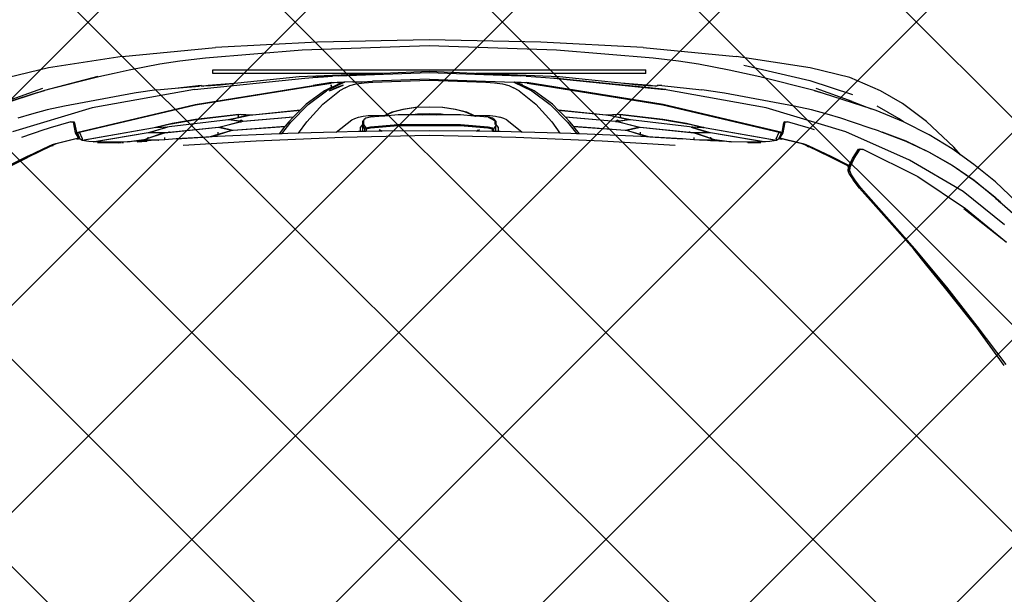
# Model space of a CAD drawing. Units: inches. Extents: x 2167 to 2589, y 1680 to 2489.
# Tile 27 of 38: x 2356 to 2389, y 1815 to 1835. Entities that reach past the tile are written whole.
import ezdxf

# ---------------------------------------------------------------- set-up
doc = ezdxf.new("R2010")
doc.units = ezdxf.units.IN
doc.header["$MEASUREMENT"] = 0
doc.layers.get('0').update_dxf_attribs({"color": 250})
doc.layers.add('C-PRKG-VEHS', color=8, linetype='Continuous', lineweight=13)
doc.layers.add('L-PVMT-PATT', color=252, linetype='Continuous', lineweight=13)
doc.layers.add('Edges', color=250, linetype='Continuous')

# ---------------------------------------------------------------- blocks, each defined once
blk = doc.blocks.new('Nissan Qashqai pl')
at = {"layer": 'Edges'}
for p, q in [((7.4801, 12.6274), (7.4565, 12.6023)), ((7.4827, 12.6103), (7.5001, 12.6302)), ((7.5081, 12.6131), (7.4679, 12.5634)), ((7.4884, 12.5664), (7.5289, 12.6158)), ((7.5243, 12.6101), (7.5286, 12.6146)), ((7.676, 12.6152), (7.6296, 12.5803)), ((7.6769, 12.6129), (7.6306, 12.5791)), ((7.4565, 12.6023), (7.4354, 12.5766)), ((7.4542, 12.5765), (7.4744, 12.6015)), ((7.475, 12.6016), (7.4549, 12.5767)), ((7.4744, 12.6015), (7.4804, 12.6079)), ((7.4762, 12.6028), (7.475, 12.6016)), ((7.4752, 12.6016), (7.4762, 12.6028)), ((7.4762, 12.6028), (7.478, 12.6049)), ((7.4804, 12.6079), (7.478, 12.6049)), ((7.478, 12.6049), (7.479, 12.6061)), ((7.479, 12.6061), (7.4815, 12.6089)), ((7.479, 12.6061), (7.4801, 12.6074)), ((7.4801, 12.6074), (7.4804, 12.6079)), ((7.4804, 12.6079), (7.4807, 12.6082)), ((7.4804, 12.6079), (7.4804, 12.6079)), ((7.4807, 12.6082), (7.4821, 12.6097)), ((7.4815, 12.6089), (7.4821, 12.6097)), ((7.4821, 12.6097), (7.4827, 12.6103)), ((7.4882, 12.5645), (7.5243, 12.6101)), ((7.4354, 12.5766), (7.4239, 12.5604)), ((7.4363, 12.5502), (7.4542, 12.5765)), ((7.4549, 12.5767), (7.4369, 12.5504)), ((7.6296, 12.5803), (7.5827, 12.5441)), ((7.6301, 12.5787), (7.618, 12.5691)), ((7.6306, 12.5791), (7.6301, 12.5787)), ((7.4498, 12.5093), (7.4884, 12.5664)), ((7.618, 12.5691), (7.5829, 12.5411)), ((7.618, 12.5691), (7.584, 12.5429)), ((7.4147, 12.5524), (7.3837, 12.5197)), ((7.4239, 12.5604), (7.4147, 12.5524)), ((7.4239, 12.5604), (7.4166, 12.5503)), ((7.4679, 12.5634), (7.4302, 12.4993)), ((7.4166, 12.5503), (7.3997, 12.5227)), ((7.4205, 12.5229), (7.4363, 12.5502)), ((7.4369, 12.5504), (7.4211, 12.5232)), ((7.5827, 12.5441), (7.5369, 12.5057)), ((7.584, 12.5429), (7.5568, 12.5201)), ((7.5829, 12.5411), (7.5568, 12.5201)), ((7.3837, 12.5197), (7.3624, 12.4907)), ((7.3997, 12.5227), (7.3845, 12.4925)), ((7.4071, 12.4948), (7.4205, 12.5229)), ((7.4211, 12.5232), (7.4078, 12.4951)), ((7.5568, 12.5201), (7.5371, 12.5042)), ((7.4172, 12.4431), (7.4498, 12.5093)), ((7.5369, 12.5057), (7.4635, 12.4408)), ((7.3962, 12.466), (7.4071, 12.4948)), ((7.4302, 12.4993), (7.3963, 12.4227)), ((7.4078, 12.4951), (7.3969, 12.4665)), ((7.4638, 12.439), (7.5371, 12.5042)), ((7.3624, 12.4907), (7.347, 12.4644)), ((7.3805, 12.4866), (7.3655, 12.4604)), ((7.3843, 12.492), (7.3707, 12.4592)), ((7.3843, 12.492), (7.3805, 12.4866)), ((7.3845, 12.4925), (7.3843, 12.492)), ((7.347, 12.4644), (7.3309, 12.4276)), ((7.3707, 12.4592), (7.3688, 12.4532)), ((7.3938, 12.4583), (7.3925, 12.4542)), ((7.3951, 12.462), (7.3938, 12.4583)), ((7.3965, 12.4655), (7.3951, 12.462)), ((7.3965, 12.4655), (7.3962, 12.466)), ((7.3969, 12.4665), (7.3965, 12.4655)), ((7.3968, 12.4649), (7.3967, 12.4651)), ((7.3688, 12.4532), (7.3467, 12.3846)), ((7.3596, 12.4302), (7.3688, 12.4532)), ((7.3925, 12.4542), (7.3845, 12.4306)), ((7.4167, 12.4393), (7.4169, 12.4406)), ((7.4167, 12.4393), (7.4172, 12.4395)), ((7.417, 12.4377), (7.4167, 12.4393)), ((7.4169, 12.4412), (7.4172, 12.4431)), ((7.4169, 12.4406), (7.4172, 12.4423)), ((7.4169, 12.4406), (7.4169, 12.4412)), ((7.4169, 12.4398), (7.4169, 12.4406)), ((7.4282, 12.4328), (7.4169, 12.4398)), ((7.4172, 12.4395), (7.4169, 12.4398)), ((7.4283, 12.4307), (7.417, 12.4377)), ((7.4172, 12.4423), (7.4174, 12.4429)), ((7.4183, 12.4382), (7.4172, 12.4395)), ((7.4175, 12.4429), (7.4174, 12.4429)), ((7.4183, 12.4382), (7.4296, 12.4312)), ((7.4635, 12.4408), (7.4541, 12.4333)), ((7.4638, 12.439), (7.4541, 12.4313)), ((7.3309, 12.4276), (7.3193, 12.3797)), ((7.3345, 12.3793), (7.3514, 12.4308)), ((7.3596, 12.4302), (7.344, 12.3869)), ((7.3963, 12.4227), (7.3676, 12.3269)), ((7.3845, 12.4306), (7.3799, 12.4164)), ((7.4255, 12.4044), (7.4367, 12.4268)), ((7.4365, 12.4235), (7.4267, 12.4041)), ((7.4387, 12.428), (7.4282, 12.4328)), ((7.4359, 12.4272), (7.4283, 12.4307)), ((7.4383, 12.4272), (7.4296, 12.4312)), ((7.4367, 12.4268), (7.4359, 12.4272)), ((7.4378, 12.4261), (7.4365, 12.4235)), ((7.4365, 12.4235), (7.4365, 12.4235)), ((7.4367, 12.4268), (7.4383, 12.4272)), ((7.4379, 12.4263), (7.4378, 12.4261)), ((7.4379, 12.4263), (7.4383, 12.4272)), ((7.4379, 12.4263), (7.4389, 12.4269)), ((7.4384, 12.426), (7.4379, 12.4263)), ((7.4384, 12.426), (7.438, 12.4251)), ((7.4383, 12.4272), (7.4389, 12.4269)), ((7.4389, 12.4269), (7.4384, 12.426)), ((7.4387, 12.4259), (7.4384, 12.426)), ((7.4431, 12.4276), (7.4387, 12.428)), ((7.443, 12.4254), (7.4387, 12.4259)), ((7.44, 12.4264), (7.4389, 12.4269)), ((7.44, 12.4264), (7.4442, 12.4258)), ((7.4477, 12.427), (7.443, 12.4254)), ((7.4479, 12.4293), (7.4431, 12.4276)), ((7.4442, 12.4258), (7.4477, 12.427)), ((7.4477, 12.427), (7.4541, 12.4313)), ((7.4541, 12.4333), (7.4479, 12.4293)), ((7.3799, 12.4164), (7.375, 12.4)), ((7.375, 12.4), (7.3699, 12.3813)), ((7.4131, 12.3783), (7.4255, 12.4044)), ((7.4267, 12.4041), (7.4139, 12.3778)), ((7.3467, 12.3846), (7.3489, 12.3925)), ((7.3193, 12.3797), (7.3059, 12.291)), ((7.3161, 12.3001), (7.3345, 12.3793)), ((7.3467, 12.3846), (7.33, 12.3192)), ((7.3699, 12.3813), (7.3653, 12.3604)), ((7.3913, 12.3774), (7.3844, 12.3526)), ((7.3913, 12.3774), (7.3914, 12.3775)), ((7.3925, 12.3813), (7.3914, 12.3775)), ((7.3937, 12.3851), (7.3925, 12.3813)), ((7.4115, 12.3746), (7.4131, 12.3783)), ((7.4139, 12.3778), (7.4122, 12.3742)), ((7.4133, 12.3759), (7.4142, 12.3776)), ((7.4033, 12.3435), (7.4101, 12.3708)), ((7.4108, 12.3703), (7.4042, 12.3435)), ((7.4101, 12.3708), (7.4115, 12.3746)), ((7.4122, 12.3742), (7.4108, 12.3703)), ((7.3653, 12.3604), (7.3497, 12.2767)), ((7.3841, 12.3485), (7.3844, 12.3526)), ((7.3971, 12.3461), (7.3635, 12.2033)), ((7.364, 12.2029), (7.3968, 12.3424)), ((7.3846, 12.3495), (7.3841, 12.3485)), ((7.3841, 12.3485), (7.3853, 12.3483)), ((7.3846, 12.3495), (7.3976, 12.347)), ((7.3971, 12.3461), (7.3853, 12.3483)), ((7.3968, 12.3424), (7.398, 12.3449)), ((7.4046, 12.3389), (7.3968, 12.3424)), ((7.3983, 12.3458), (7.3971, 12.3461)), ((7.3976, 12.347), (7.4026, 12.3439)), ((7.398, 12.3449), (7.3999, 12.344)), ((7.398, 12.3449), (7.4012, 12.3441)), ((7.4012, 12.3441), (7.3983, 12.3458)), ((7.3999, 12.344), (7.4051, 12.3415)), ((7.3999, 12.344), (7.4048, 12.3417)), ((7.4033, 12.3427), (7.4012, 12.3441)), ((7.4012, 12.3441), (7.4015, 12.344)), ((7.4015, 12.344), (7.4028, 12.3437)), ((7.4026, 12.3439), (7.4033, 12.3435)), ((7.4033, 12.3435), (7.4042, 12.3422)), ((7.4042, 12.3422), (7.4033, 12.3427)), ((7.4042, 12.3435), (7.404, 12.3429)), ((7.404, 12.3429), (7.4043, 12.3428)), ((7.404, 12.3429), (7.4043, 12.3425)), ((7.4041, 12.3435), (7.4042, 12.3435)), ((7.4042, 12.3435), (7.4045, 12.3434)), ((7.4042, 12.3422), (7.4043, 12.3425)), ((7.4044, 12.3422), (7.4042, 12.3422)), ((7.4043, 12.3428), (7.4045, 12.3434)), ((7.4043, 12.3428), (7.4046, 12.3425)), ((7.4043, 12.3425), (7.4043, 12.3428)), ((7.4043, 12.3425), (7.4044, 12.3422)), ((7.4044, 12.3422), (7.4046, 12.3419)), ((7.4046, 12.3422), (7.4044, 12.3422)), ((7.4045, 12.3434), (7.405, 12.3456)), ((7.4045, 12.3434), (7.4048, 12.3433)), ((7.4046, 12.3425), (7.4047, 12.3424)), ((7.4047, 12.3424), (7.4046, 12.3422)), ((7.4046, 12.3422), (7.4046, 12.3419)), ((7.4048, 12.3422), (7.4046, 12.3422)), ((7.4046, 12.3419), (7.405, 12.3419)), ((7.4048, 12.3417), (7.4046, 12.3419)), ((7.4047, 12.3424), (7.4048, 12.3422)), ((7.4048, 12.3422), (7.405, 12.3419)), ((7.4048, 12.3417), (7.4052, 12.3416)), ((7.4051, 12.3415), (7.4048, 12.3417)), ((7.405, 12.3419), (7.4052, 12.3416)), ((7.4051, 12.3415), (7.4052, 12.3415)), ((7.4052, 12.3416), (7.4052, 12.3415)), ((7.4052, 12.3415), (7.4063, 12.3395)), ((7.4062, 12.3389), (7.4063, 12.3395)), ((7.4063, 12.3395), (7.4065, 12.3392)), ((7.3916, 12.2547), (7.4062, 12.3389)), ((7.4065, 12.3392), (7.3917, 12.2547)), ((7.4046, 12.3389), (7.4062, 12.3389)), ((7.4065, 12.3392), (7.4066, 12.3389)), ((7.4066, 12.3389), (7.408, 12.3313)), ((7.408, 12.3313), (7.4083, 12.3258)), ((7.33, 12.3192), (7.3261, 12.3009)), ((7.3676, 12.3269), (7.3455, 12.2042)), ((7.3971, 12.2599), (7.4083, 12.3258)), ((7.4084, 12.3244), (7.3975, 12.2599)), ((7.4083, 12.3258), (7.4084, 12.3244)), ((7.4084, 12.3244), (7.4087, 12.3195)), ((7.4087, 12.3195), (7.4087, 12.3037)), ((7.4092, 12.3184), (7.4091, 12.3206)), ((7.4092, 12.305), (7.4092, 12.3184)), ((7.3261, 12.3009), (7.3223, 12.2825)), ((7.4087, 12.3037), (7.4081, 12.2848)), ((7.2951, 12.1791), (7.3059, 12.291)), ((7.3223, 12.2825), (7.3186, 12.2641)), ((7.4054, 12.2651), (7.4081, 12.2848)), ((7.4081, 12.2838), (7.4079, 12.2798)), ((7.4081, 12.2848), (7.4081, 12.2838)), ((7.3494, 12.2741), (7.3457, 12.2495)), ((7.3498, 12.2768), (7.3494, 12.2741)), ((7.3497, 12.2767), (7.3494, 12.2741)), ((7.4079, 12.2798), (7.4059, 12.2651)), ((7.4079, 12.2798), (7.4069, 12.2598)), ((7.3186, 12.2641), (7.3149, 12.2457)), ((7.391, 12.2387), (7.3967, 12.2579)), ((7.3969, 12.257), (7.3965, 12.256)), ((7.3967, 12.2579), (7.3971, 12.2599)), ((7.3968, 12.2559), (7.3969, 12.257)), ((7.3975, 12.2599), (7.3973, 12.258)), ((7.3973, 12.258), (7.3977, 12.2439)), ((7.4048, 12.2612), (7.3982, 12.2419)), ((7.3983, 12.244), (7.4038, 12.2599)), ((7.4028, 12.2599), (7.4038, 12.2599)), ((7.4038, 12.2599), (7.4049, 12.2631)), ((7.4053, 12.2622), (7.4048, 12.2612)), ((7.4049, 12.2631), (7.4054, 12.2651)), ((7.4053, 12.2612), (7.4053, 12.2622)), ((7.4061, 12.2473), (7.4053, 12.2612)), ((7.4059, 12.2618), (7.4056, 12.2621)), ((7.4059, 12.2651), (7.4058, 12.2632)), ((7.4058, 12.2632), (7.4059, 12.2618)), ((7.4059, 12.2618), (7.4064, 12.2523)), ((7.4069, 12.2598), (7.4064, 12.2523)), ((7.3149, 12.2457), (7.3113, 12.2217)), ((7.3407, 12.2016), (7.3457, 12.2495)), ((7.3909, 12.2508), (7.3864, 12.231)), ((7.3869, 12.2347), (7.3912, 12.2527)), ((7.3901, 12.2368), (7.391, 12.2507)), ((7.3914, 12.2527), (7.3906, 12.2386)), ((7.3908, 12.2366), (7.3965, 12.256)), ((7.3911, 12.2518), (7.3909, 12.2508)), ((7.391, 12.2507), (7.3911, 12.2518)), ((7.3912, 12.2517), (7.3911, 12.2518)), ((7.3912, 12.2527), (7.3916, 12.2547)), ((7.3917, 12.2547), (7.3914, 12.2527)), ((7.3972, 12.2421), (7.3968, 12.2559)), ((7.4061, 12.2472), (7.4057, 12.24)), ((7.4064, 12.2523), (7.4061, 12.2473)), ((7.4061, 12.2472), (7.4061, 12.2473)), ((7.3813, 12.2021), (7.3869, 12.2347)), ((7.3815, 12.1638), (7.3899, 12.2348)), ((7.3903, 12.2347), (7.382, 12.1639)), ((7.3899, 12.2348), (7.3901, 12.2368)), ((7.3908, 12.2366), (7.3903, 12.2347)), ((7.3905, 12.1754), (7.3966, 12.2347)), ((7.3906, 12.2386), (7.3907, 12.2376)), ((7.3907, 12.2376), (7.391, 12.2387)), ((7.3977, 12.24), (7.3911, 12.1755)), ((7.3957, 12.2348), (7.3966, 12.2348)), ((7.3957, 12.2347), (7.3966, 12.2347)), ((7.3966, 12.2348), (7.3972, 12.24)), ((7.3966, 12.2347), (7.3966, 12.2348)), ((7.3972, 12.24), (7.3972, 12.2421)), ((7.3977, 12.2439), (7.398, 12.2429)), ((7.3982, 12.2419), (7.3977, 12.24)), ((7.398, 12.2429), (7.3983, 12.244)), ((7.4032, 12.24), (7.4057, 12.24)), ((7.4057, 12.24), (7.4048, 12.2262)), ((7.3113, 12.2217), (7.3078, 12.191)), ((7.3864, 12.231), (7.3815, 12.2029)), ((7.4022, 12.187), (7.4048, 12.2262)), ((7.4048, 12.2262), (7.4023, 12.1836)), ((7.4072, 12.1299), (7.4124, 12.2176)), ((7.3455, 12.2062), (7.3317, 12.0717)), ((7.3317, 12.0717), (7.3455, 12.2042)), ((7.3407, 12.2016), (7.34, 12.1962)), ((7.3403, 12.1981), (7.3407, 12.2016)), ((7.3635, 12.2033), (7.3405, 12.0616)), ((7.3426, 12.0707), (7.364, 12.2029)), ((7.375, 12.1484), (7.3813, 12.2021)), ((7.3815, 12.2029), (7.3756, 12.1509)), ((7.3078, 12.191), (7.298, 12.075)), ((7.3407, 12.1879), (7.3378, 12.1521)), ((7.34, 12.1962), (7.3401, 12.1962)), ((7.3401, 12.1962), (7.341, 12.1962)), ((7.3413, 12.1933), (7.3407, 12.1879)), ((7.341, 12.1962), (7.3414, 12.1962)), ((7.341, 12.1962), (7.341, 12.1962)), ((7.3414, 12.1962), (7.341, 12.1962)), ((7.341, 12.1962), (7.3413, 12.1933)), ((7.3413, 12.1931), (7.341, 12.1848)), ((7.3415, 12.1954), (7.3413, 12.1933)), ((7.3413, 12.1933), (7.3413, 12.1931)), ((7.4017, 12.185), (7.4022, 12.187)), ((7.2951, 12.1791), (7.2884, 12.0562)), ((7.3261, 12.1821), (7.3216, 12.1821)), ((7.3216, 11.6621), (7.3216, 12.1821)), ((7.3261, 12.1821), (7.3261, 11.9779)), ((7.341, 12.1848), (7.34, 12.1731)), ((7.3901, 12.1734), (7.3905, 12.1754)), ((7.3911, 12.1755), (7.3913, 12.1737)), ((7.3949, 12.1616), (7.399, 12.1756)), ((7.4021, 12.1833), (7.3951, 12.1606)), ((7.3967, 12.1756), (7.399, 12.1756)), ((7.4018, 12.1764), (7.3986, 12.1025)), ((7.399, 12.1756), (7.4017, 12.185)), ((7.4023, 12.1836), (7.4018, 12.1764)), ((7.4023, 12.1836), (7.4021, 12.1833)), ((7.34, 12.1731), (7.3378, 12.1521)), ((7.3792, 12.1518), (7.3812, 12.1619)), ((7.3812, 12.1619), (7.3815, 12.1638)), ((7.382, 12.1639), (7.382, 12.1619)), ((7.382, 12.1619), (7.3838, 12.1497)), ((7.3843, 12.1498), (7.3877, 12.1639)), ((7.3903, 12.1716), (7.3844, 12.1479)), ((7.3877, 12.1639), (7.3874, 12.1639)), ((7.3877, 12.1639), (7.3901, 12.1734)), ((7.3907, 12.1727), (7.3903, 12.1716)), ((7.3909, 12.1716), (7.3907, 12.1727)), ((7.3939, 12.1596), (7.3909, 12.1716)), ((7.3913, 12.1737), (7.3943, 12.1614)), ((7.3378, 12.1521), (7.3302, 12.0785)), ((7.3756, 12.1509), (7.3792, 12.1518)), ((7.3756, 12.1509), (7.3762, 12.138)), ((7.3813, 12.1599), (7.3763, 12.1361)), ((7.3764, 12.138), (7.3792, 12.1518)), ((7.3815, 12.161), (7.3813, 12.1599)), ((7.3817, 12.16), (7.3815, 12.161)), ((7.3832, 12.1493), (7.3817, 12.16)), ((7.3896, 12.0954), (7.3941, 12.1576)), ((7.3945, 12.1577), (7.3903, 12.0959)), ((7.3941, 12.1576), (7.3939, 12.1596)), ((7.3943, 12.1614), (7.3947, 12.1605)), ((7.3951, 12.1606), (7.3945, 12.1577)), ((7.3947, 12.1605), (7.3949, 12.1616)), ((7.376, 12.136), (7.375, 12.1484)), ((7.3783, 12.0852), (7.3836, 12.1459)), ((7.384, 12.1459), (7.3788, 12.0857)), ((7.3832, 12.1493), (7.3824, 12.1487)), ((7.3824, 12.1487), (7.3832, 12.1492)), ((7.3836, 12.1459), (7.3824, 12.1487)), ((7.3824, 12.1487), (7.3835, 12.1468)), ((7.3838, 12.1497), (7.3832, 12.1493)), ((7.3832, 12.1492), (7.3837, 12.1495)), ((7.3832, 12.1492), (7.3832, 12.1493)), ((7.3836, 12.1459), (7.3835, 12.1468)), ((7.3835, 12.1468), (7.384, 12.1459)), ((7.3837, 12.1495), (7.3843, 12.1498)), ((7.3837, 12.1495), (7.3838, 12.1497)), ((7.384, 12.1459), (7.3842, 12.1495)), ((7.3844, 12.1479), (7.384, 12.1459)), ((7.3842, 12.1495), (7.3843, 12.1498)), ((7.3843, 12.1495), (7.3842, 12.1495)), ((7.3701, 12.0771), (7.3759, 12.1341)), ((7.3761, 12.1341), (7.3704, 12.0773)), ((7.3759, 12.1341), (7.376, 12.136)), ((7.3763, 12.1361), (7.3761, 12.1341)), ((7.3762, 12.137), (7.3764, 12.138)), ((7.3762, 12.138), (7.3762, 12.137)), ((7.3764, 12.1371), (7.3762, 12.137)), ((7.4025, 12.026), (7.4072, 12.1299)), ((7.3841, 12.091), (7.3788, 12.0857)), ((7.3896, 12.0954), (7.3841, 12.091)), ((7.3845, 12.0883), (7.3985, 12.0993)), ((7.3903, 12.0959), (7.3896, 12.0954)), ((7.3986, 12.1025), (7.3903, 12.0959)), ((7.3982, 12.092), (7.3978, 12.0791)), ((7.3985, 12.0993), (7.3982, 12.092)), ((7.3986, 12.1025), (7.3985, 12.0993)), ((7.3633, 12.0674), (7.3845, 12.0883)), ((7.3783, 12.0852), (7.3704, 12.0773)), ((7.3788, 12.0857), (7.3783, 12.0852)), ((7.3842, 12.0693), (7.3978, 12.0791)), ((7.3978, 12.0791), (7.3966, 12.0338)), ((7.298, 12.075), (7.2928, 11.9221)), ((7.3302, 12.0785), (7.3261, 11.9779)), ((7.3309, 12.0619), (7.3317, 12.0717)), ((7.341, 12.0605), (7.3426, 12.0707)), ((7.3631, 12.0701), (7.3469, 12.0481)), ((7.3471, 12.0454), (7.3633, 12.0674)), ((7.363, 12.0501), (7.3842, 12.0693)), ((7.3701, 12.0771), (7.3631, 12.0701)), ((7.3704, 12.0773), (7.3701, 12.0771)), ((7.2884, 12.0562), (7.2857, 11.9221)), ((7.3294, 12.0385), (7.3309, 12.0619)), ((7.3405, 12.0616), (7.3369, 12.0394)), ((7.3377, 12.0398), (7.341, 12.0605)), ((7.3365, 12.0237), (7.3471, 12.0454)), ((7.3469, 12.0481), (7.3402, 12.0337)), ((7.3468, 12.0299), (7.363, 12.0501)), ((7.3294, 12.0385), (7.3291, 12.0316)), ((7.3362, 12.0248), (7.3365, 12.0321)), ((7.3365, 12.0321), (7.3369, 12.0394)), ((7.3377, 12.0398), (7.3369, 12.0328)), ((7.3369, 12.0287), (7.3369, 12.0328)), ((7.3402, 12.0337), (7.338, 12.0291)), ((7.3387, 12.0332), (7.3402, 12.0337)), ((7.3818, 12.0151), (7.3966, 12.0338)), ((7.3966, 12.0338), (7.3959, 12.0071)), ((7.3251, 11.9221), (7.3291, 12.0316)), ((7.3329, 11.9221), (7.3365, 12.0237)), ((7.3362, 12.0248), (7.3366, 12.0246)), ((7.3365, 12.0237), (7.3362, 12.0248)), ((7.338, 12.0291), (7.3369, 12.0287)), ((7.3374, 12.0276), (7.3369, 12.0287)), ((7.338, 12.0291), (7.3374, 12.0276)), ((7.3407, 12.0176), (7.3432, 12.0231)), ((7.3468, 12.0299), (7.3432, 12.0231)), ((7.4002, 11.9221), (7.4025, 12.026)), ((7.3373, 12.0004), (7.3386, 12.01)), ((7.3386, 12.01), (7.3407, 12.0176)), ((7.3801, 12.0115), (7.3786, 12.007)), ((7.3818, 12.0151), (7.3801, 12.0115)), ((7.3367, 11.99), (7.3373, 12.0004)), ((7.3768, 11.9954), (7.3775, 12.0015)), ((7.3775, 12.0015), (7.3786, 12.007)), ((7.3798, 11.9983), (7.3787, 11.9928)), ((7.3808, 11.9993), (7.3798, 11.9983)), ((7.3807, 11.9991), (7.3798, 11.9983)), ((7.38, 11.9953), (7.383, 12.0011)), ((7.3807, 11.9991), (7.3808, 11.9993)), ((7.381, 11.9993), (7.3807, 11.9991)), ((7.3808, 11.9993), (7.384, 12.0021)), ((7.381, 11.9993), (7.3808, 11.9993)), ((7.383, 12.0011), (7.381, 11.9993)), ((7.3866, 12.0011), (7.383, 12.0011)), ((7.384, 12.0021), (7.387, 12.0021)), ((7.3868, 12.002), (7.3866, 12.0011)), ((7.3875, 12.0011), (7.3866, 12.0011)), ((7.387, 12.0021), (7.3868, 12.002)), ((7.3909, 12.0051), (7.387, 12.0021)), ((7.387, 12.0021), (7.3885, 12.0021)), ((7.3885, 12.0021), (7.3925, 11.9993)), ((7.3955, 12.0021), (7.3885, 12.0021)), ((7.3904, 11.9928), (7.3916, 11.9983)), ((7.3956, 12.0051), (7.3909, 12.0051)), ((7.3929, 11.9981), (7.3917, 11.9926)), ((7.3925, 11.9993), (7.3958, 11.9993)), ((7.3925, 11.9993), (7.3929, 11.9981)), ((7.3958, 11.9981), (7.3929, 11.9981)), ((7.3955, 12.0021), (7.3958, 12.0018)), ((7.3959, 12.0049), (7.3956, 12.0051)), ((7.3959, 12.0051), (7.3956, 12.0051)), ((7.3958, 11.9981), (7.3956, 11.9801)), ((7.3959, 12.0049), (7.3958, 12.0018)), ((7.3958, 12.0018), (7.3958, 11.9993)), ((7.3958, 11.9993), (7.3958, 11.9981)), ((7.3959, 12.0071), (7.3959, 12.0051)), ((7.3959, 12.0051), (7.3959, 12.0049)), ((7.3343, 11.9221), (7.3367, 11.99)), ((7.3761, 11.9751), (7.3765, 11.989)), ((7.3765, 11.989), (7.3768, 11.9954)), ((7.3787, 11.9928), (7.3774, 11.9778)), ((7.3787, 11.9928), (7.38, 11.9953)), ((7.3876, 11.9595), (7.3904, 11.9928)), ((7.3917, 11.9926), (7.3889, 11.9594)), ((7.3261, 11.9764), (7.3238, 11.9221)), ((7.3261, 11.9764), (7.3261, 11.9779)), ((7.3724, 11.9667), (7.3761, 11.9751)), ((7.3771, 11.9757), (7.3727, 11.9658)), ((7.3773, 11.9759), (7.3759, 11.9595)), ((7.3761, 11.9751), (7.3769, 11.9767)), ((7.3769, 11.9767), (7.3771, 11.977)), ((7.3774, 11.9778), (7.3771, 11.9771)), ((7.3771, 11.9771), (7.3774, 11.9774)), ((7.3771, 11.9771), (7.3771, 11.977)), ((7.3773, 11.9759), (7.3771, 11.9757)), ((7.3774, 11.9774), (7.3773, 11.9759)), ((7.3774, 11.9774), (7.3774, 11.9778)), ((7.3938, 11.9823), (7.3956, 11.9801)), ((7.3956, 11.9788), (7.3938, 11.981)), ((7.3956, 11.9788), (7.3951, 11.9221)), ((7.3956, 11.9801), (7.3956, 11.9788)), ((7.369, 11.9536), (7.3724, 11.9667)), ((7.3727, 11.9658), (7.3693, 11.953)), ((7.3668, 11.9384), (7.369, 11.9536)), ((7.3693, 11.953), (7.3672, 11.9381)), ((7.3759, 11.9595), (7.3759, 11.9417)), ((7.3876, 11.8847), (7.3876, 11.9595)), ((7.3889, 11.9594), (7.3889, 11.8848)), ((7.3661, 11.9221), (7.3668, 11.9384)), ((7.3672, 11.9381), (7.3665, 11.9221)), ((7.3759, 11.9417), (7.3751, 11.9363)), ((7.3759, 11.9417), (7.3759, 11.9303)), ((7.3751, 11.9363), (7.3745, 11.9221)), ((7.3755, 11.9221), (7.3759, 11.9303)), ((7.3759, 11.9303), (7.3759, 11.9139)), ((7.2857, 11.9221), (7.2884, 11.7879)), ((7.2928, 11.9221), (7.298, 11.7692)), ((7.3238, 11.9221), (7.3261, 11.8662)), ((7.3291, 11.8126), (7.3251, 11.9221)), ((7.3329, 11.9221), (7.3354, 11.8539)), ((7.3367, 11.8541), (7.3343, 11.9221)), ((7.3668, 11.9057), (7.3661, 11.9221)), ((7.3665, 11.9221), (7.3672, 11.9061)), ((7.3745, 11.9221), (7.3751, 11.9078)), ((7.3759, 11.9139), (7.3755, 11.9221)), ((7.3759, 11.9139), (7.3759, 11.9025)), ((7.3951, 11.9221), (7.3956, 11.8653)), ((7.4025, 11.8181), (7.4002, 11.9221)), ((7.369, 11.8905), (7.3668, 11.9057)), ((7.3672, 11.9061), (7.3693, 11.8911)), ((7.3751, 11.9078), (7.3759, 11.9025)), ((7.3759, 11.9025), (7.3759, 11.8847)), ((7.3724, 11.8775), (7.369, 11.8905)), ((7.3693, 11.8911), (7.3727, 11.8783)), ((7.3727, 11.8783), (7.3771, 11.8685)), ((7.3759, 11.8847), (7.3773, 11.8682)), ((7.3904, 11.8513), (7.3876, 11.8847)), ((7.3889, 11.8848), (7.3917, 11.8516)), ((7.3261, 11.8662), (7.3302, 11.7656)), ((7.3261, 11.8662), (7.3261, 11.6621)), ((7.3761, 11.8691), (7.3724, 11.8775)), ((7.3765, 11.8551), (7.3761, 11.8691)), ((7.3769, 11.8674), (7.3761, 11.8691)), ((7.3771, 11.8671), (7.3769, 11.8674)), ((7.3771, 11.8685), (7.3773, 11.8682)), ((7.3771, 11.8671), (7.3771, 11.8671)), ((7.3771, 11.8671), (7.3774, 11.8664)), ((7.3774, 11.8668), (7.3771, 11.8671)), ((7.3773, 11.8682), (7.3774, 11.8668)), ((7.3774, 11.8668), (7.3774, 11.8664)), ((7.3774, 11.8664), (7.3787, 11.8513)), ((7.3768, 11.8488), (7.3765, 11.8551)), ((7.3938, 11.8632), (7.3956, 11.8653)), ((7.3956, 11.864), (7.3938, 11.8619)), ((7.3956, 11.8653), (7.3956, 11.864)), ((7.3956, 11.864), (7.3958, 11.8461)), ((7.3361, 11.8416), (7.3354, 11.8539)), ((7.3373, 11.8438), (7.3367, 11.8541)), ((7.3386, 11.8342), (7.3373, 11.8438)), ((7.3775, 11.8427), (7.3768, 11.8488)), ((7.3786, 11.8372), (7.3775, 11.8427)), ((7.3787, 11.8513), (7.3798, 11.8459)), ((7.3798, 11.8459), (7.3808, 11.8448)), ((7.3808, 11.8448), (7.3807, 11.8451)), ((7.3808, 11.8448), (7.381, 11.8448)), ((7.384, 11.8421), (7.3808, 11.8448)), ((7.383, 11.8431), (7.3875, 11.8431)), ((7.3875, 11.8431), (7.3916, 11.8459)), ((7.3925, 11.8448), (7.3885, 11.8421)), ((7.3916, 11.8459), (7.3904, 11.8513)), ((7.3917, 11.8516), (7.3929, 11.8461)), ((7.3929, 11.8461), (7.3925, 11.8448)), ((7.3958, 11.8448), (7.3925, 11.8448)), ((7.3929, 11.8461), (7.3958, 11.8461)), ((7.3958, 11.8461), (7.3958, 11.8448)), ((7.3958, 11.8448), (7.3958, 11.8423)), ((7.3362, 11.8301), (7.3361, 11.8416)), ((7.3407, 11.8266), (7.3386, 11.8342)), ((7.3801, 11.8327), (7.3786, 11.8372)), ((7.3818, 11.8291), (7.3801, 11.8327)), ((7.387, 11.8421), (7.384, 11.8421)), ((7.387, 11.8421), (7.3909, 11.8391)), ((7.3885, 11.8421), (7.387, 11.8421)), ((7.3955, 11.8421), (7.3885, 11.8421)), ((7.3909, 11.8391), (7.3956, 11.8391)), ((7.3958, 11.8423), (7.3955, 11.8421)), ((7.3956, 11.8391), (7.3959, 11.8392)), ((7.3956, 11.8391), (7.3959, 11.8391)), ((7.3958, 11.8423), (7.3959, 11.8392)), ((7.3959, 11.8392), (7.3959, 11.8391)), ((7.3959, 11.8391), (7.3959, 11.8371)), ((7.3959, 11.8371), (7.3966, 11.8103)), ((7.3362, 11.8301), (7.3365, 11.8204)), ((7.3362, 11.8194), (7.3365, 11.8204)), ((7.3367, 11.8196), (7.3362, 11.8194)), ((7.3365, 11.812), (7.3362, 11.8194)), ((7.3365, 11.8204), (7.3471, 11.7987)), ((7.3432, 11.821), (7.3407, 11.8266)), ((7.3432, 11.821), (7.3468, 11.8142)), ((7.3966, 11.8103), (7.3818, 11.8291)), ((7.3291, 11.8126), (7.3294, 11.8057)), ((7.3369, 11.8047), (7.3365, 11.812)), ((7.3369, 11.8155), (7.3374, 11.8165)), ((7.3369, 11.8113), (7.3369, 11.8155)), ((7.3369, 11.8155), (7.338, 11.8151)), ((7.3369, 11.8113), (7.3377, 11.8044)), ((7.3374, 11.8165), (7.338, 11.8151)), ((7.338, 11.8151), (7.343, 11.8045)), ((7.3401, 11.8186), (7.3431, 11.8112)), ((7.347, 11.8021), (7.3401, 11.8186)), ((7.3431, 11.8112), (7.347, 11.8021)), ((7.363, 11.794), (7.3468, 11.8142)), ((7.3966, 11.8103), (7.3978, 11.7651)), ((7.4072, 11.7142), (7.4025, 11.8181)), ((7.3301, 11.7949), (7.3294, 11.8057)), ((7.3295, 11.8012), (7.3309, 11.7822)), ((7.3295, 11.8012), (7.3301, 11.7949)), ((7.3369, 11.8047), (7.3405, 11.7825)), ((7.3377, 11.8042), (7.3377, 11.8044)), ((7.341, 11.7837), (7.3377, 11.8042)), ((7.343, 11.8045), (7.3396, 11.8043)), ((7.3396, 11.8043), (7.3431, 11.8042)), ((7.343, 11.8045), (7.3431, 11.8042)), ((7.3431, 11.8042), (7.3469, 11.7961)), ((7.3469, 11.7961), (7.3631, 11.774)), ((7.3633, 11.7767), (7.3471, 11.7987)), ((7.2884, 11.7879), (7.2951, 11.6651)), ((7.3309, 11.7822), (7.3301, 11.7949)), ((7.3426, 11.7735), (7.341, 11.7837)), ((7.3842, 11.7749), (7.363, 11.794)), ((7.3317, 11.7724), (7.3309, 11.7822)), ((7.3455, 11.64), (7.3317, 11.7724)), ((7.3635, 11.6409), (7.3405, 11.7825)), ((7.364, 11.6413), (7.3426, 11.7735)), ((7.3631, 11.774), (7.3701, 11.7671)), ((7.3845, 11.7558), (7.3633, 11.7767)), ((7.3978, 11.7651), (7.3842, 11.7749)), ((7.298, 11.7692), (7.3078, 11.6532)), ((7.3302, 11.7656), (7.3378, 11.6921)), ((7.3759, 11.7101), (7.3701, 11.7671)), ((7.3701, 11.7671), (7.3704, 11.7668)), ((7.3704, 11.7668), (7.3761, 11.71)), ((7.3704, 11.7668), (7.3783, 11.759)), ((7.3978, 11.7651), (7.3982, 11.7521)), ((7.3836, 11.6983), (7.3783, 11.759)), ((7.3783, 11.759), (7.3788, 11.7585)), ((7.3788, 11.7585), (7.384, 11.6982)), ((7.3788, 11.7585), (7.3841, 11.7532)), ((7.3841, 11.7532), (7.3896, 11.7488)), ((7.3985, 11.7448), (7.3845, 11.7558)), ((7.3941, 11.6865), (7.3896, 11.7488)), ((7.3896, 11.7488), (7.3903, 11.7483)), ((7.3903, 11.7483), (7.3945, 11.6865)), ((7.3903, 11.7483), (7.3986, 11.7417)), ((7.3982, 11.7521), (7.3985, 11.7448)), ((7.3985, 11.7448), (7.3986, 11.7417)), ((7.3986, 11.7417), (7.4018, 11.6678)), ((7.4124, 11.6265), (7.4072, 11.7142)), ((7.375, 11.6957), (7.376, 11.7081)), ((7.3762, 11.7062), (7.3757, 11.6959)), ((7.376, 11.7081), (7.3759, 11.7101)), ((7.3761, 11.71), (7.3763, 11.7081)), ((7.3762, 11.7062), (7.3764, 11.7061)), ((7.3763, 11.7081), (7.3813, 11.6842)), ((7.3764, 11.7061), (7.3792, 11.6924)), ((7.3378, 11.6921), (7.3407, 11.6563)), ((7.3378, 11.6921), (7.34, 11.671)), ((7.3813, 11.642), (7.375, 11.6957)), ((7.3757, 11.6959), (7.3756, 11.6933)), ((7.3792, 11.6924), (7.3756, 11.6933)), ((7.3756, 11.6933), (7.3815, 11.6413)), ((7.3757, 11.6959), (7.3757, 11.6959)), ((7.3812, 11.6823), (7.3792, 11.6924)), ((7.3817, 11.6844), (7.3832, 11.6949)), ((7.3838, 11.6944), (7.382, 11.6823)), ((7.3824, 11.6955), (7.3836, 11.6983)), ((7.3835, 11.6973), (7.3824, 11.6955)), ((7.3834, 11.6959), (7.3824, 11.6955)), ((7.3824, 11.6955), (7.3832, 11.6949)), ((7.3832, 11.695), (7.3824, 11.6955)), ((7.3832, 11.695), (7.3834, 11.6959)), ((7.3838, 11.6947), (7.3832, 11.695)), ((7.3832, 11.6949), (7.3838, 11.6944)), ((7.3837, 11.696), (7.3834, 11.6959)), ((7.3835, 11.6973), (7.3836, 11.6983)), ((7.3836, 11.6975), (7.3835, 11.6973)), ((7.3836, 11.6975), (7.3836, 11.6983)), ((7.384, 11.6982), (7.3836, 11.6975)), ((7.3844, 11.6963), (7.3837, 11.696)), ((7.3838, 11.6947), (7.3837, 11.696)), ((7.3843, 11.6944), (7.3838, 11.6947)), ((7.3843, 11.6942), (7.3838, 11.6944)), ((7.3843, 11.6944), (7.3844, 11.6963)), ((7.3843, 11.6942), (7.3843, 11.6944)), ((7.3877, 11.6803), (7.3843, 11.6942)), ((7.3844, 11.6963), (7.3903, 11.6725)), ((7.3815, 11.6804), (7.3812, 11.6823)), ((7.3813, 11.6842), (7.3817, 11.6844)), ((7.3817, 11.6841), (7.3813, 11.6842)), ((7.3899, 11.6094), (7.3815, 11.6804)), ((7.3817, 11.6841), (7.3817, 11.6844)), ((7.382, 11.6823), (7.382, 11.6803)), ((7.382, 11.6803), (7.3903, 11.6095)), ((7.3874, 11.6803), (7.3877, 11.6803)), ((7.3901, 11.6707), (7.3877, 11.6803)), ((7.3909, 11.6728), (7.3939, 11.6846)), ((7.3943, 11.6827), (7.3913, 11.6705)), ((7.3939, 11.6846), (7.3941, 11.6865)), ((7.3943, 11.6827), (7.3949, 11.6826)), ((7.3943, 11.6827), (7.395, 11.6825)), ((7.3945, 11.6865), (7.3951, 11.6835)), ((7.395, 11.6825), (7.3949, 11.6826)), ((7.399, 11.6686), (7.395, 11.6825)), ((7.3951, 11.6835), (7.4021, 11.6609)), ((7.3059, 11.5532), (7.2951, 11.6651)), ((7.34, 11.671), (7.341, 11.6594)), ((7.3905, 11.6687), (7.3901, 11.6707)), ((7.3909, 11.6728), (7.3903, 11.6725)), ((7.3909, 11.6725), (7.3903, 11.6725)), ((7.3966, 11.6095), (7.3905, 11.6687)), ((7.3909, 11.6725), (7.3909, 11.6728)), ((7.3913, 11.6705), (7.3911, 11.6687)), ((7.3911, 11.6687), (7.3977, 11.6042)), ((7.399, 11.6686), (7.3967, 11.6686)), ((7.4017, 11.6592), (7.399, 11.6686)), ((7.4018, 11.6678), (7.4022, 11.6609)), ((7.3261, 11.6621), (7.3216, 11.6621)), ((7.3407, 11.6563), (7.3413, 11.6509)), ((7.341, 11.6594), (7.3413, 11.6511)), ((7.4022, 11.6571), (7.4017, 11.6592)), ((7.4022, 11.6609), (7.4021, 11.6609)), ((7.4022, 11.6609), (7.4021, 11.6609)), ((7.4022, 11.6609), (7.4048, 11.618)), ((7.4022, 11.6609), (7.4022, 11.6609)), ((7.4048, 11.618), (7.4022, 11.6571)), ((7.3078, 11.6532), (7.3113, 11.6224)), ((7.3401, 11.648), (7.34, 11.648)), ((7.3438, 11.6167), (7.34, 11.648)), ((7.341, 11.648), (7.3401, 11.648)), ((7.341, 11.648), (7.3413, 11.6509)), ((7.3414, 11.648), (7.341, 11.648)), ((7.341, 11.648), (7.3414, 11.648)), ((7.3438, 11.6167), (7.3412, 11.646)), ((7.3413, 11.6511), (7.3413, 11.6509)), ((7.3413, 11.6509), (7.3415, 11.6488)), ((7.3869, 11.6094), (7.3813, 11.642)), ((7.3455, 11.64), (7.3676, 11.5172)), ((7.3971, 11.4981), (7.3635, 11.6409)), ((7.3968, 11.5018), (7.364, 11.6413)), ((7.3815, 11.6413), (7.3864, 11.6131)), ((7.3113, 11.6224), (7.3149, 11.5984)), ((7.4048, 11.618), (7.4057, 11.6042)), ((7.3457, 11.5947), (7.3438, 11.6167)), ((7.3864, 11.6131), (7.3909, 11.5933)), ((7.3912, 11.5914), (7.3869, 11.6094)), ((7.3901, 11.6073), (7.3899, 11.6094)), ((7.391, 11.5935), (7.3901, 11.6073)), ((7.3903, 11.6095), (7.3908, 11.6076)), ((7.3908, 11.6076), (7.3965, 11.5881)), ((7.3966, 11.6095), (7.3957, 11.6095)), ((7.3972, 11.6042), (7.3966, 11.6095)), ((7.3149, 11.5984), (7.3186, 11.58)), ((7.3457, 11.5947), (7.3494, 11.57)), ((7.3906, 11.6055), (7.391, 11.6055)), ((7.3906, 11.6055), (7.391, 11.6054)), ((7.3906, 11.6055), (7.3914, 11.5914)), ((7.391, 11.6054), (7.391, 11.6055)), ((7.3967, 11.5862), (7.391, 11.6054)), ((7.3968, 11.5882), (7.3972, 11.6021)), ((7.3972, 11.6021), (7.3972, 11.6042)), ((7.3977, 11.6003), (7.3973, 11.5862)), ((7.3977, 11.6042), (7.3982, 11.6022)), ((7.3977, 11.6003), (7.3983, 11.6002)), ((7.3977, 11.6003), (7.3983, 11.6001)), ((7.3982, 11.6022), (7.4048, 11.5829)), ((7.3983, 11.6001), (7.3983, 11.6002)), ((7.4038, 11.5843), (7.3983, 11.6001)), ((7.4057, 11.6042), (7.4032, 11.6042)), ((7.4053, 11.5831), (7.4061, 11.5969)), ((7.4057, 11.6042), (7.4061, 11.597)), ((7.4061, 11.5969), (7.4061, 11.597)), ((7.4061, 11.5969), (7.4064, 11.5919)), ((7.391, 11.5935), (7.3909, 11.5933)), ((7.391, 11.5934), (7.3909, 11.5933)), ((7.3916, 11.5894), (7.3912, 11.5914)), ((7.3914, 11.5914), (7.3917, 11.5895)), ((7.4062, 11.5053), (7.3916, 11.5894)), ((7.3917, 11.5895), (7.4065, 11.505)), ((7.3968, 11.5882), (7.3965, 11.5881)), ((7.3971, 11.5842), (7.3967, 11.5862)), ((7.3968, 11.5882), (7.3973, 11.5884)), ((7.4083, 11.5184), (7.3971, 11.5842)), ((7.3973, 11.5862), (7.3975, 11.5843)), ((7.3975, 11.5843), (7.4084, 11.5198)), ((7.4038, 11.5843), (7.4028, 11.5843)), ((7.4049, 11.5811), (7.4038, 11.5843)), ((7.4053, 11.5831), (7.4048, 11.5829)), ((7.4053, 11.583), (7.4048, 11.5829)), ((7.406, 11.5834), (7.4053, 11.5831)), ((7.406, 11.5833), (7.4053, 11.583)), ((7.4053, 11.583), (7.4053, 11.5831)), ((7.406, 11.5833), (7.4058, 11.581)), ((7.4064, 11.5919), (7.406, 11.5834)), ((7.406, 11.5834), (7.406, 11.5833)), ((7.4064, 11.5919), (7.4069, 11.5844)), ((7.4069, 11.5844), (7.4079, 11.5644)), ((7.4081, 11.5711), (7.4075, 11.5828)), ((7.3186, 11.58), (7.3223, 11.5616)), ((7.4054, 11.5791), (7.4049, 11.5811)), ((7.4081, 11.5593), (7.4054, 11.5791)), ((7.4058, 11.581), (7.4059, 11.579)), ((7.4059, 11.579), (7.4079, 11.5644)), ((7.3223, 11.5616), (7.3261, 11.5433)), ((7.3494, 11.57), (7.3497, 11.5674)), ((7.3494, 11.57), (7.3498, 11.5674)), ((7.3497, 11.5674), (7.3653, 11.4838)), ((7.4079, 11.5644), (7.4081, 11.5604)), ((7.4079, 11.5644), (7.4081, 11.5629)), ((7.4081, 11.5604), (7.4081, 11.5593)), ((7.4081, 11.5593), (7.4087, 11.5405)), ((7.3059, 11.5532), (7.3193, 11.4645)), ((7.4092, 11.5416), (7.409, 11.5485)), ((7.4096, 11.549), (7.4092, 11.5521)), ((7.4093, 11.5546), (7.4095, 11.5529)), ((7.3261, 11.5433), (7.33, 11.5249)), ((7.4087, 11.5405), (7.4087, 11.5246)), ((7.4092, 11.5258), (7.4092, 11.5416)), ((7.3297, 11.5237), (7.3467, 11.4596)), ((7.33, 11.5249), (7.3467, 11.4596)), ((7.4087, 11.5246), (7.4084, 11.5198)), ((7.4091, 11.5235), (7.4092, 11.5258)), ((7.3676, 11.5172), (7.3963, 11.4215)), ((7.408, 11.5129), (7.4066, 11.5052)), ((7.4083, 11.5184), (7.408, 11.5129)), ((7.4084, 11.5198), (7.4083, 11.5184)), ((7.4046, 11.5053), (7.3968, 11.5018)), ((7.398, 11.4993), (7.3968, 11.5018)), ((7.4026, 11.5002), (7.3976, 11.4971)), ((7.398, 11.4993), (7.4048, 11.5024)), ((7.4012, 11.5001), (7.398, 11.4993)), ((7.3983, 11.4983), (7.4012, 11.5001)), ((7.4012, 11.5001), (7.4033, 11.5014)), ((7.403, 11.5005), (7.4026, 11.5002)), ((7.403, 11.5005), (7.4028, 11.5004)), ((7.4033, 11.5007), (7.403, 11.5005)), ((7.4033, 11.5014), (7.4042, 11.502)), ((7.4042, 11.502), (7.4033, 11.5007)), ((7.4033, 11.5005), (7.4033, 11.5007)), ((7.4034, 11.5005), (7.4033, 11.5005)), ((7.4101, 11.4733), (7.4033, 11.5005)), ((7.4043, 11.5016), (7.404, 11.5012)), ((7.4043, 11.5014), (7.404, 11.5012)), ((7.404, 11.5012), (7.4108, 11.4738)), ((7.4042, 11.502), (7.4044, 11.502)), ((7.4043, 11.5016), (7.4042, 11.502)), ((7.4044, 11.502), (7.4043, 11.5016)), ((7.4046, 11.5016), (7.4043, 11.5014)), ((7.4043, 11.5014), (7.4043, 11.5016)), ((7.4045, 11.5008), (7.4043, 11.5014)), ((7.4046, 11.5023), (7.4044, 11.502)), ((7.4044, 11.502), (7.4046, 11.502)), ((7.4048, 11.5008), (7.4045, 11.5008)), ((7.405, 11.4985), (7.4045, 11.5008)), ((7.4062, 11.5053), (7.4046, 11.5053)), ((7.4046, 11.5023), (7.4048, 11.5024)), ((7.405, 11.5023), (7.4046, 11.5023)), ((7.4046, 11.5023), (7.4046, 11.502)), ((7.4046, 11.502), (7.4047, 11.5018)), ((7.4046, 11.502), (7.4048, 11.502)), ((7.4047, 11.5018), (7.4046, 11.5016)), ((7.4048, 11.502), (7.4047, 11.5018)), ((7.4048, 11.5024), (7.4052, 11.5027)), ((7.4052, 11.5026), (7.4048, 11.5024)), ((7.405, 11.5023), (7.4048, 11.502)), ((7.4052, 11.5026), (7.405, 11.5023)), ((7.4063, 11.5047), (7.4052, 11.5027)), ((7.4052, 11.5027), (7.4052, 11.5026)), ((7.4063, 11.5047), (7.4062, 11.5053)), ((7.4065, 11.505), (7.4063, 11.5047)), ((7.4066, 11.5052), (7.4065, 11.505)), ((7.3853, 11.4958), (7.3841, 11.4956)), ((7.3844, 11.4916), (7.3841, 11.4956)), ((7.3846, 11.4946), (7.3844, 11.4916)), ((7.3844, 11.4916), (7.3914, 11.4667)), ((7.3976, 11.4971), (7.3846, 11.4946)), ((7.3853, 11.4958), (7.3846, 11.4946)), ((7.3853, 11.4958), (7.3971, 11.4981)), ((7.3971, 11.4981), (7.3983, 11.4983)), ((7.3653, 11.4838), (7.3699, 11.4629)), ((7.3193, 11.4645), (7.3309, 11.4166)), ((7.3914, 11.4667), (7.3925, 11.4629)), ((7.4115, 11.4695), (7.4101, 11.4733)), ((7.4108, 11.4738), (7.4122, 11.47)), ((7.4131, 11.4659), (7.4115, 11.4695)), ((7.4122, 11.47), (7.4139, 11.4664)), ((7.4126, 11.47), (7.4125, 11.4702)), ((7.4132, 11.4685), (7.4126, 11.47)), ((7.4255, 11.4398), (7.4131, 11.4659)), ((7.4139, 11.4664), (7.4267, 11.4401)), ((7.344, 11.4572), (7.3596, 11.4139)), ((7.3489, 11.4517), (7.3467, 11.4596)), ((7.3467, 11.4596), (7.3686, 11.3913)), ((7.3699, 11.4629), (7.375, 11.4442)), ((7.3925, 11.4629), (7.3937, 11.4591)), ((7.3937, 11.4591), (7.4029, 11.4321)), ((7.3489, 11.4517), (7.3686, 11.3913)), ((7.375, 11.4442), (7.3799, 11.4278)), ((7.4255, 11.4398), (7.4367, 11.4174)), ((7.4379, 11.4179), (7.4267, 11.4401))]:
    blk.add_line(p, q, dxfattribs=at)
blk = doc.blocks.new('car')
blk.add_blockref('Nissan Qashqai pl', (-9.7433, -11.9151))
blk = doc.blocks.new('carr')
blk.add_blockref('car', (0.5124, -0.007))

msp = doc.modelspace()

# ---------------------------------------------------------------- hatches: boundary and pattern name
at = {"layer": 'L-PVMT-PATT'}
h = msp.add_hatch(dxfattribs=at)
h.set_pattern_fill('ANSI37', color=256, scale=40)
h.paths.add_polyline_path([(2417.548, 1783.695), (2417.548, 1846.042), (2239.361, 1846.042), (2239.361, 1687.695), (2369.843, 1687.695), (2369.843, 1696.695), (2375.607, 1696.695), (2416.107, 1696.695), (2417.548, 1696.695)])

# ---------------------------------------------------------------- block references
at = {"layer": 'C-PRKG-VEHS', "xscale": 28.42784210623918, "yscale": 28.42784210623918, "zscale": 28.42784210623918, "rotation": 270}
msp.add_blockref('carr', (2369.852, 1779.037), dxfattribs=at)

doc.saveas('drawing.dxf')
